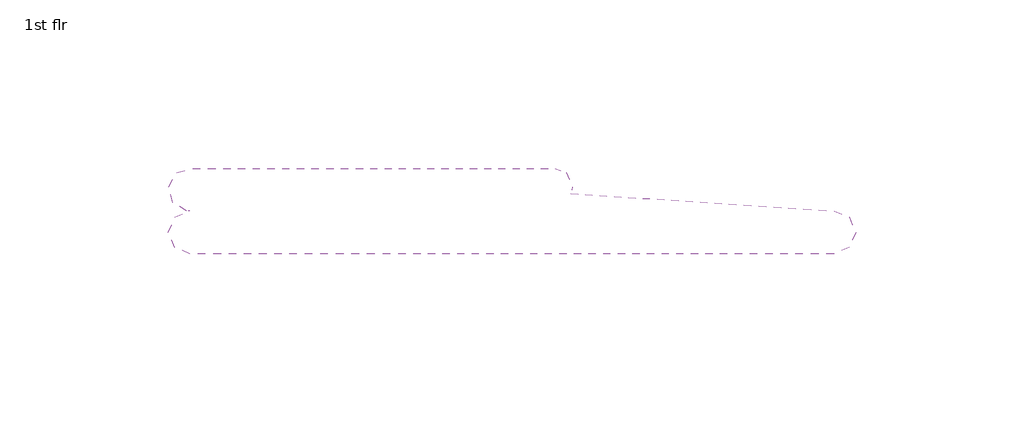
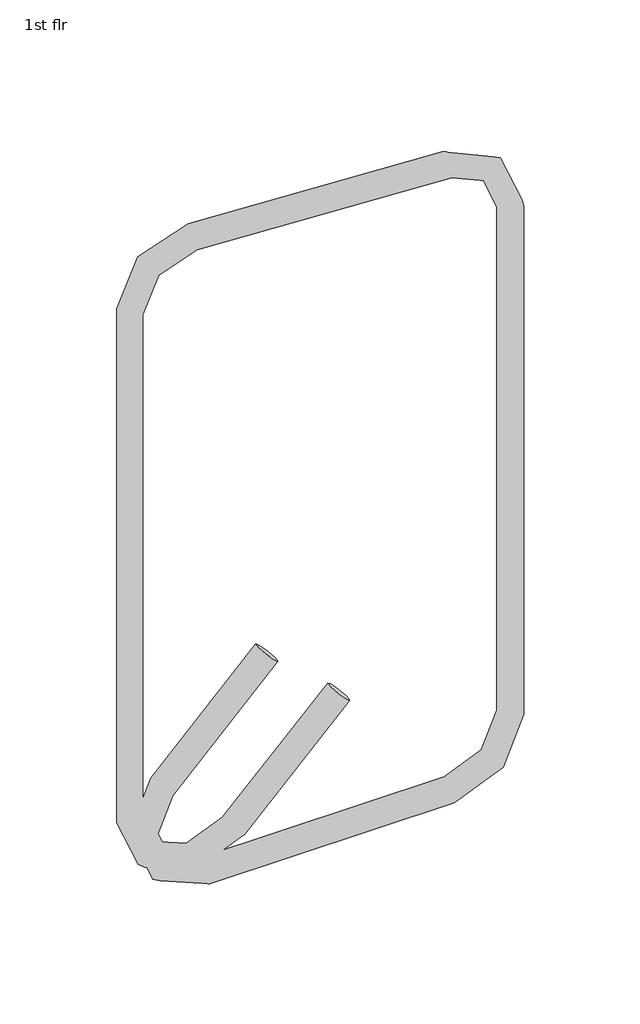
# One storey, part 2 of 2: 1 reinforcing bar.
"""IFC4 building model written with IfcOpenShell, lengths in millimetres."""

from ifc_helpers import new_model, si_unit, point, frame, origin, place, context, project, spatial, polyline, circle_curve, trimmed, segment, composite_curve, element, save
from ifc_brep_helpers import swept_disk

model = new_model("IFC4")

# Units and contexts
model_context = context("Model", 3, world=origin())
ifc_project = project(units=[si_unit("LENGTHUNIT", "METRE", prefix="MILLI")], contexts=[model_context])

# Site, building, storey
site = spatial("IfcSite", under=ifc_project)
building = spatial("IfcBuilding", under=site)
storey = spatial("IfcBuildingStorey", under=building, Name="1st flr", Elevation=3200.4)

# Reinforcing bar
placement = place(None, origin())
element("IfcReinforcingBar", 1, at=placement, inside=storey, context=model_context, shape_type="SolidModel", body=[
    swept_disk(composite_curve([segment(polyline([(-7897.6815591, 7487.9699494, 6134.8187638), (-7952.5465576, 7487.9699494, 6079.9537653)]), True, "CONTINUOUS"), segment(trimmed(circle_curve(frame((-7930.0959173, 7487.9699494, 6057.503125), z_axis=(0.0, -1.0, 0.0), x_axis=(-22.450640299999577, 0.0, 22.450640299999577)), 31.75), [point((-7952.5465576, 7487.9699494, 6079.9537653))], [point((-7930.0959173, 7487.9699494, 6025.753125))], True, "CARTESIAN"), True, "CONTINUOUS"), segment(polyline([(-7930.0959173, 7487.9699494, 6025.753125), (-7802.3021673, 7487.9699494, 6025.753125)]), True, "CONTINUOUS"), segment(trimmed(circle_curve(frame((-7802.3021673, 7487.9699494, 6057.503125), z_axis=(0.0, -1.0, 0.0), x_axis=(0.0, 0.0, -31.75)), 31.75), [point((-7802.3021673, 7487.9699494, 6025.753125))], [point((-7770.5521673, 7487.9699494, 6057.503125))], True, "CARTESIAN"), True, "CONTINUOUS"), segment(polyline([(-7770.5521673, 7487.9699494, 6057.503125), (-7770.5521673, 7487.9699494, 6337.696875)]), True, "CONTINUOUS"), segment(trimmed(circle_curve(frame((-7802.2324265, 7490.0732031, 6337.696875), z_axis=(-0.06624421176864148, -0.9978034397651431, 0.0), x_axis=(31.680259199999455, -2.1032537000000957, 0.0)), 31.75), [point((-7770.5521673, 7487.9699494, 6337.696875))], [point((-7802.2324265, 7490.0732031, 6369.446875))], True, "CARTESIAN"), True, "CONTINUOUS"), segment(polyline([(-7802.2324265, 7490.0732031, 6369.446875), (-7930.165658, 7498.5666957, 6369.446875)]), True, "CONTINUOUS"), segment(trimmed(circle_curve(frame((-7930.165658, 7498.5666957, 6337.696875), z_axis=(-0.06624421176864148, -0.9978034397651431, 0.0), x_axis=(0.0, 0.0, 31.75)), 31.75), [point((-7930.165658, 7498.5666957, 6369.446875))], [point((-7961.8459173, 7500.6699494, 6337.696875))], True, "CARTESIAN"), True, "CONTINUOUS"), segment(polyline([(-7961.8459173, 7500.6699494, 6337.696875), (-7961.8459173, 7500.6699494, 6057.503125)]), True, "CONTINUOUS"), segment(trimmed(circle_curve(frame((-7930.0959173, 7500.6699494, 6057.503125), z_axis=(0.0, -1.0, 0.0), x_axis=(-31.75, 0.0, 0.0)), 31.75), [point((-7961.8459173, 7500.6699494, 6057.503125))], [point((-7907.645277, 7500.6699494, 6035.0524847))], True, "CARTESIAN"), True, "CONTINUOUS"), segment(polyline([(-7907.645277, 7500.6699494, 6035.0524847), (-7852.7802785, 7500.6699494, 6089.9174832)]), True, "CONTINUOUS")], self_intersect=False), 6.35),
])

save(model, "model.ifc")

# Revit data of these elements
# Element 1 (IfcReinforcingBar)
#   Phase Created = New Construction
